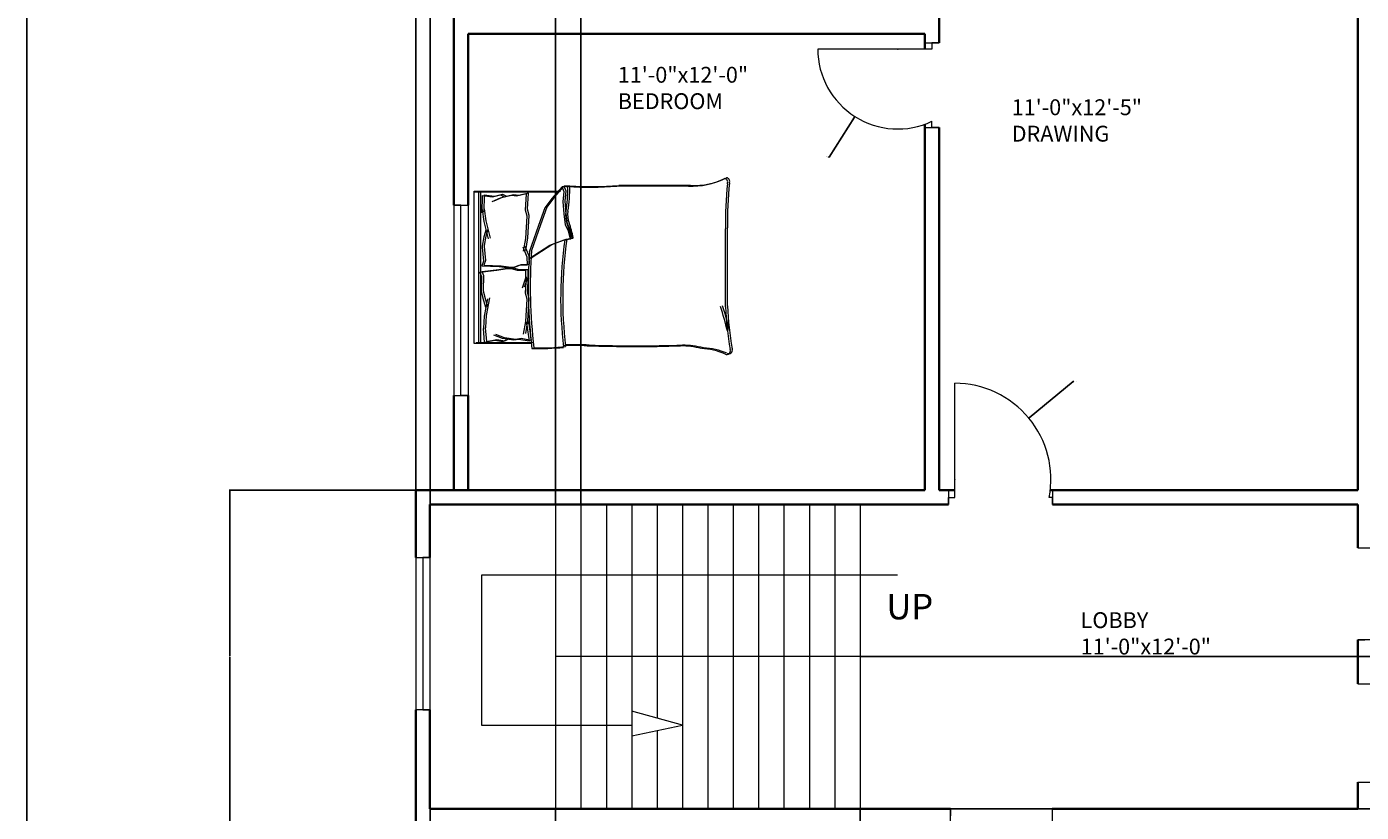
# Model space of a CAD drawing. Units: inches. Extents: x 2163 to 2982, y 1024 to 2288.
# Tile 9 of 22: x 2163 to 2583, y 1637 to 1885. Entities that reach past the tile are written whole.
import ezdxf

# ---------------------------------------------------------------- set-up
doc = ezdxf.new("R2010")
doc.units = ezdxf.units.IN
for name, color, linetype, lineweight in [('A-ANNO-DIMS', 2, 'Continuous', 18), ('A-ANNO-SYMB', 81, 'Continuous', 18), ('A-ANNO-TEXT', 7, 'Continuous', 18), ('A-ANNO-TTLB', 7, 'Continuous', 25), ('A-AREA-IDEN', 7, 'Continuous', 18), ('A-DOOR', 11, 'Continuous', 18), ('A-FLOR-STRS', 81, 'Continuous', 18), ('A-FURN', 8, 'Continuous', 13), ('A-GLAZ', 161, 'Continuous', 18), ('A-WALL', 7, 'Continuous', 35)]:
    doc.layers.add(name, color=color, linetype=linetype, lineweight=lineweight)
doc.styles.get("Standard").update_dxf_attribs({"font": 'arial.ttf'})
doc.dimstyles.get("Standard").update_dxf_attribs({"dimtxt": 0.18, "dimasz": 0.18, "dimexe": 0.18, "dimexo": 0.0625, "dimgap": 0.09, "dimtad": 0, "dimtih": 1, "dimtoh": 1, "dimdec": 4, "dimzin": 0, "dimdsep": 46, "dimtxsty": 'Standard', "dimcen": 0.09, "dimadec": 0, "dimazin": 0, "dimtfac": 1, "dimtdec": 4, "dimtofl": 0, "dimtmove": 0, "dimatfit": 3, "dimfxl": 1, "dimtolj": 1, "dimtzin": 0, "dimarcsym": 0})

# ---------------------------------------------------------------- blocks, each defined once
blk = doc.blocks.new('BED-DOUBLE')
for p, q in [((0, 51.49), (0.64, 51.49)), ((0, 3.47), (0, 51.49)), ((0, 51.27), (26.61, 51.27)), ((0, 51.27), (26.61, 51.27)), ((0.64, 51.49), (27.25, 51.49)), ((0.64, 51.49), (27.25, 51.49)), ((1.53, 3.48), (1.53, 51.27)), ((1.53, 3.47), (1.53, 51.27)), ((2.17, 3.7), (2.17, 51.49)), ((2.17, 3.7), (2.17, 51.49)), ((6.41, 49.96), (8.98, 50.56)), ((6.41, 49.96), (8.98, 50.56)), ((8.98, 50.56), (10.02, 50.04)), ((8.98, 50.56), (10.02, 50.04)), ((16.57, 50.7), (13.43, 49.92)), ((16.57, 50.7), (13.43, 49.92)), ((17.21, 50.93), (14.07, 50.15)), ((17.21, 50.93), (14.07, 50.15)), ((16.17, 45.57), (16.57, 50.7)), ((16.17, 45.57), (16.57, 50.7)), ((16.81, 45.79), (17.21, 50.93)), ((16.81, 45.79), (17.21, 50.93)), ((27.75, 52.87), (24.5, 49.16)), ((27.75, 52.87), (24.5, 49.16)), ((28.38, 53.1), (25.13, 49.39)), ((28.38, 53.1), (25.13, 49.39)), ((29.49, 52.95), (27.75, 52.87, 3.87)), ((29.49, 52.95), (27.75, 52.87, 3.87)), ((28.36, 51.33), (27.75, 52.87)), ((28.36, 51.33), (27.75, 52.87)), ((28.06, 48.23), (28.36, 51.33)), ((28.06, 48.23), (28.36, 51.33)), ((30.13, 53.18), (28.38, 53.1, 3.87)), ((29, 51.56), (28.38, 53.1)), ((30.13, 53.18), (28.38, 53.1, 3.87)), ((29, 51.56), (28.38, 53.1)), ((28.69, 48.46), (29, 51.56)), ((28.69, 48.46), (29, 51.56)), ((2.56, 50.11), (2.46, 44.71)), ((2.56, 50.11), (2.46, 44.71)), ((2.56, 50.11), (5.77, 49.73)), ((2.56, 50.11), (5.77, 49.73)), ((3.2, 50.34), (3.1, 44.94)), ((3.2, 50.34), (3.1, 44.94)), ((3.2, 50.34), (6.41, 49.96)), ((3.2, 50.34), (6.41, 49.96)), ((8.26, 49.31), (5.58, 48.13)), ((8.26, 49.31), (5.58, 48.13)), ((5.77, 49.73), (8.34, 50.33)), ((5.77, 49.73), (8.34, 50.33)), ((8.9, 49.54), (6.22, 48.36)), ((8.9, 49.54), (6.22, 48.36)), ((11.83, 50.11), (8.26, 49.31)), ((11.83, 50.11), (8.26, 49.31)), ((8.34, 50.33), (9.38, 49.81)), ((8.34, 50.33), (9.38, 49.81)), ((12.47, 50.34), (8.9, 49.54)), ((12.47, 50.34), (8.9, 49.54)), ((13.43, 49.92), (11.83, 50.11)), ((13.43, 49.92), (11.83, 50.11)), ((14.07, 50.15), (12.47, 50.34)), ((14.07, 50.15), (12.47, 50.34)), ((22.97, 46.45), (20.96, 40.87)), ((22.97, 46.45), (20.96, 40.87)), ((24.5, 49.16), (22.33, 46.22)), ((24.5, 49.16), (22.33, 46.22)), ((25.13, 49.39), (22.97, 46.45)), ((25.13, 49.39), (22.97, 46.45)), ((28.36, 44.36), (28.06, 48.23)), ((28.36, 44.36), (28.06, 48.23)), ((29, 44.59), (28.69, 48.46)), ((29, 44.59), (28.69, 48.46)), ((2.46, 44.71), (2.54, 45.71)), ((2.46, 44.71), (2.54, 45.71)), ((2.54, 45.71), (3.07, 41.91)), ((2.54, 45.71), (3.07, 41.91)), ((3.1, 44.94), (3.18, 45.94)), ((3.1, 44.94), (3.18, 45.94)), ((3.18, 45.94), (3.71, 42.14)), ((3.18, 45.94), (3.71, 42.14)), ((3.71, 42.14), (5.06, 36.72)), ((3.71, 42.14), (5.06, 36.72)), ((16.73, 43.61), (16.17, 45.57)), ((16.73, 43.61), (16.17, 45.57)), ((16.29, 36.6), (16.73, 43.61)), ((16.29, 36.6), (16.73, 43.61)), ((17.37, 43.83), (16.81, 45.79)), ((17.37, 43.83), (16.81, 45.79)), ((16.93, 36.82), (17.37, 43.83)), ((16.93, 36.82), (17.37, 43.83)), ((22.33, 46.22), (20.32, 40.64)), ((22.33, 46.22), (20.32, 40.64)), ((28.83, 40.95), (28.36, 44.36)), ((28.83, 40.95), (28.36, 44.36)), ((29.47, 41.18), (29, 44.59)), ((29.47, 41.18), (29, 44.59)), ((3.07, 41.91), (4.42, 36.49)), ((3.07, 41.91), (4.42, 36.49)), ((3.67, 39.2), (3.08, 37.14)), ((3.67, 39.2), (3.08, 37.13)), ((4.31, 39.43), (3.72, 37.36)), ((4.31, 39.43), (3.72, 37.36)), ((20.32, 40.64), (17.38, 32.31)), ((20.32, 40.64), (17.38, 32.31)), ((20.96, 40.87), (18.02, 32.53)), ((20.96, 40.87), (18.02, 32.53)), ((29.76, 38.94), (28.83, 40.95)), ((29.76, 38.94), (28.83, 40.95)), ((30.4, 39.17), (29.47, 41.18)), ((30.4, 39.17), (29.47, 41.18)), ((30.38, 36.46), (29.76, 38.94)), ((30.38, 36.46), (29.76, 38.94)), ((31.02, 36.69), (30.4, 39.17)), ((31.02, 36.69), (30.4, 39.17)), ((79.24, 15.06), (79.24, 39.68)), ((79.24, 15.06), (79.24, 39.68)), ((79.88, 15.29), (79.88, 39.91)), ((79.88, 15.29), (79.88, 39.91)), ((3.08, 37.14), (2.54, 34.2)), ((3.08, 37.13), (2.54, 34.2)), ((2.54, 34.2), (2.56, 33.88)), ((2.54, 34.2), (2.56, 33.88)), ((2.56, 33.88), (2.98, 29.46)), ((2.56, 33.88), (2.98, 29.46)), ((3.72, 37.36), (3.18, 34.43)), ((3.72, 37.36), (3.18, 34.43)), ((3.18, 34.43), (3.2, 34.11)), ((3.18, 34.43), (3.2, 34.11)), ((3.2, 34.11), (3.62, 29.68)), ((3.2, 34.11), (3.62, 29.68)), ((16.74, 30.75), (15.45, 33.82)), ((16.74, 30.75), (15.45, 33.82)), ((15.63, 32.56), (16.29, 36.6)), ((15.63, 32.56), (16.29, 36.6)), ((17.38, 30.98), (16.09, 34.05)), ((17.38, 30.98), (16.09, 34.05)), ((16.27, 32.79), (16.93, 36.82)), ((16.27, 32.79), (16.93, 36.82)), ((17.38, 30.26), (23.88, 34.45)), ((17.38, 30.26), (23.88, 34.45)), ((18.02, 30.49), (24.52, 34.68)), ((18.02, 30.49), (24.52, 34.68)), ((23.88, 34.45), (28.36, 36.15)), ((23.88, 34.45), (28.36, 36.15)), ((24.52, 34.68), (29, 36.38)), ((24.52, 34.68), (29, 36.38)), ((28.36, 36.15), (30.38, 36.46)), ((28.36, 36.15), (30.38, 36.46)), ((29, 36.38), (31.02, 36.69)), ((29, 36.38), (31.02, 36.69)), ((2.98, 29.46), (2.49, 27.98)), ((2.98, 29.46), (2.49, 27.98)), ((3.62, 29.68), (3.13, 28.21)), ((3.62, 29.68), (3.13, 28.2)), ((16.89, 28.3), (16.74, 30.75)), ((16.89, 28.3), (16.74, 30.75)), ((17.53, 28.53), (17.38, 30.98)), ((17.53, 28.53), (17.38, 30.98)), ((1.87, 25.98), (7.22, 26.56)), ((1.87, 25.98), (7.22, 26.56)), ((2.45, 24.54), (1.87, 25.98)), ((2.45, 24.54), (1.87, 25.98)), ((2.49, 27.98), (7.87, 27.73)), ((2.49, 27.98), (7.87, 27.73)), ((2.51, 26.21), (7.86, 26.79)), ((2.51, 26.21), (7.86, 26.79)), ((3.09, 24.77), (2.51, 26.21)), ((3.09, 24.77), (2.51, 26.21)), ((3.13, 28.21), (8.51, 27.96)), ((3.13, 28.2), (8.51, 27.96)), ((7.22, 26.56), (10.4, 27.14)), ((7.22, 26.56), (10.4, 27.14)), ((7.86, 26.79), (11.04, 27.37)), ((7.86, 26.79), (11.04, 27.37)), ((7.87, 27.73), (11.08, 27.35)), ((7.87, 27.73), (11.08, 27.35)), ((8.51, 27.96), (11.72, 27.58)), ((8.51, 27.96), (11.72, 27.58)), ((10.4, 27.14), (11.7, 27.14)), ((10.4, 27.14), (11.7, 27.14)), ((11.04, 27.37), (12.34, 27.37)), ((11.04, 27.37), (12.34, 27.37)), ((11.08, 27.35), (12.38, 27.44)), ((11.08, 27.35), (12.38, 27.44)), ((11.7, 27.14), (13.58, 26.56)), ((11.7, 27.14), (13.58, 26.56)), ((11.72, 27.58), (13.02, 27.66)), ((11.72, 27.58), (13.02, 27.66)), ((12.34, 27.37), (14.22, 26.79)), ((12.34, 27.37), (14.22, 26.79)), ((12.38, 27.44), (14.22, 28.13)), ((12.38, 27.44), (14.22, 28.13)), ((13.02, 27.66), (14.86, 28.36)), ((13.02, 27.66), (14.86, 28.36)), ((13.58, 26.56), (16.26, 26.56)), ((13.58, 26.56), (16.26, 26.56)), ((14.22, 28.13), (16.89, 28.3)), ((14.22, 28.13), (16.89, 28.3)), ((14.22, 26.79), (16.9, 26.79)), ((14.22, 26.79), (16.9, 26.79)), ((14.86, 28.36), (17.53, 28.53)), ((14.86, 28.36), (17.53, 28.53)), ((16.26, 26.56), (16.26, 24.1)), ((16.26, 26.56), (16.26, 24.1)), ((16.9, 26.79), (16.9, 24.33)), ((16.9, 26.79), (16.9, 24.33)), ((2.3, 20.09), (2.45, 24.54)), ((2.3, 20.09), (2.45, 24.54)), ((2.94, 20.32), (3.09, 24.77)), ((2.94, 20.32), (3.09, 24.77)), ((16.26, 24.1), (15.17, 20.96)), ((16.26, 24.1), (15.17, 20.96)), ((16.9, 24.33), (15.81, 21.19)), ((16.9, 24.33), (15.81, 21.19)), ((16.17, 19.38), (16.57, 24.52)), ((16.17, 19.38), (16.57, 24.52)), ((16.81, 19.61), (17.21, 24.74)), ((16.81, 19.61), (17.21, 24.74)), ((2.3, 19.77), (2.3, 20.09)), ((2.3, 19.77), (2.3, 20.09)), ((3.03, 16.88), (2.3, 19.77)), ((3.03, 16.88), (2.3, 19.77)), ((2.94, 20), (2.94, 20.32)), ((2.94, 20), (2.94, 20.32)), ((3.67, 17.11), (2.94, 20)), ((3.67, 17.11), (2.94, 20)), ((3.75, 14.85), (3.03, 16.88)), ((3.75, 14.85), (3.03, 16.88)), ((3.32, 12.11), (4.33, 17.6)), ((3.32, 12.11), (4.33, 17.6)), ((4.39, 15.08), (3.67, 17.11)), ((4.39, 15.08), (3.67, 17.11)), ((3.96, 12.34), (4.97, 17.83)), ((3.96, 12.34), (4.97, 17.83)), ((16.73, 17.42), (16.17, 19.38)), ((16.73, 17.42), (16.17, 19.38)), ((16.29, 10.41), (16.73, 17.42)), ((16.29, 10.41), (16.73, 17.42)), ((17.37, 17.65), (16.81, 19.61)), ((17.37, 17.65), (16.81, 19.61)), ((16.93, 10.64), (17.37, 17.65)), ((16.93, 10.64), (17.37, 17.65)), ((3.03, 8.28), (3.32, 12.11)), ((3.03, 8.28), (3.32, 12.11)), ((3.65, 8.41), (3.67, 8.51)), ((3.65, 8.41), (3.67, 8.51)), ((3.67, 8.51), (3.96, 12.34)), ((3.67, 8.51), (3.96, 12.34)), ((15.63, 6.38), (16.29, 10.41)), ((15.63, 6.38), (16.29, 10.41)), ((16.27, 6.61), (16.93, 10.64)), ((16.27, 6.61), (16.93, 10.64)), ((16.29, 10.41), (16.62, 9.28)), ((16.29, 10.41), (16.62, 9.28)), ((16.62, 9.28), (17.34, 4.18)), ((16.62, 9.28), (17.34, 4.18)), ((16.93, 10.64), (17.26, 9.51)), ((16.93, 10.64), (17.26, 9.51)), ((17.26, 9.51), (17.98, 4.41)), ((17.26, 9.51), (17.98, 4.41)), ((3.01, 8.18), (3.03, 8.28)), ((3.01, 8.18), (3.03, 8.28)), ((3.34, 3.9), (3.01, 8.18)), ((3.34, 3.9), (3.01, 8.18)), ((3.32, 3.89), (6.5, 4.47)), ((3.32, 3.89), (6.5, 4.47)), ((3.98, 4.13), (3.65, 8.41)), ((3.98, 4.13), (3.65, 8.41)), ((3.96, 4.12), (7.14, 4.7)), ((3.96, 4.12), (7.14, 4.7)), ((8.95, 5.05), (6.21, 6.06)), ((8.95, 5.05), (6.21, 6.06)), ((6.5, 4.47), (9.1, 4.04)), ((6.5, 4.47), (9.1, 4.04)), ((9.59, 5.28), (6.85, 6.29)), ((9.59, 5.28), (6.85, 6.29)), ((7.14, 4.7), (9.74, 4.27)), ((7.14, 4.7), (9.74, 4.27)), ((12.57, 4.47), (8.95, 5.05)), ((12.57, 4.47), (8.95, 5.05)), ((9.1, 4.04), (10.11, 4.62)), ((9.1, 4.04), (10.11, 4.62)), ((13.21, 4.7), (9.59, 5.28)), ((13.21, 4.7), (9.59, 5.28)), ((9.74, 4.27), (10.75, 4.85)), ((9.74, 4.27), (10.75, 4.85)), ((14.16, 4.76), (12.57, 4.47)), ((14.16, 4.76), (12.57, 4.47)), ((14.8, 4.99), (13.21, 4.7)), ((14.8, 4.99), (13.21, 4.7)), ((17.34, 4.18), (14.16, 4.76)), ((17.34, 4.18), (14.16, 4.76)), ((17.98, 4.41), (14.8, 4.99)), ((17.98, 4.41), (14.8, 4.99)), ((18.11, 3.48), (0, 3.48)), ((18.11, 3.47), (0, 3.47)), ((18.75, 3.7), (0.64, 3.7)), ((18.75, 3.7), (0.64, 3.7))]:
    blk.add_line(p, q)
for centre, radius, start, end in [((68.67, 76.16), 23.07, 267.4714, 296.4681), ((68.67, 76.16), 23.07, 267.4714, 296.4681), ((69.31, 76.39), 23.07, 267.4714, 296.4681), ((69.31, 76.39), 23.07, 267.4714, 296.4681), ((78.87, 54.41), 1.1, 332.6588, 86.02), ((78.87, 54.41), 1.1, 332.6588, 86.02), ((79.51, 54.64), 1.1, 332.6588, 86.02), ((79.51, 54.64), 1.1, 332.6588, 86.02), ((-6.66, 51.33), 36.18, 349.8763, 2.5657), ((-6.66, 51.33), 36.18, 349.8763, 2.5657), ((36.31, 182.27), 129.5, 266.9791, 273.8365), ((36.31, 182.27), 129.5, 266.9791, 273.8365), ((-6.02, 51.56), 36.18, 349.8763, 2.5657), ((-6.02, 51.56), 36.18, 349.8763, 2.5657), ((36.95, 182.49), 129.5, 266.9791, 273.8365), ((36.95, 182.49), 129.5, 266.9791, 273.8365), ((67.82, -4508.74), 4561.86, 90.00217, 90.28689), ((67.82, -4508.74), 4561.86, 90.00217, 90.28689), ((68.46, -4508.52), 4561.86, 90.00217, 90.28689), ((68.46, -4508.52), 4561.86, 90.00217, 90.28689), ((212.28, 41.15), 133.04, 174.4998, 180.6351), ((212.28, 41.15), 133.04, 174.4998, 180.6351), ((212.92, 41.38), 133.04, 174.4998, 180.6351), ((212.92, 41.38), 133.04, 174.4998, 180.6351), ((35.07, 43.74), 6.22, 168.6608, 203.7384), ((35.07, 43.74), 6.22, 168.6608, 203.7384), ((35.71, 43.97), 6.22, 168.6608, 203.7384), ((35.71, 43.97), 6.22, 168.6608, 203.7384), ((1.48, 31.15), 29.65, 10.6617, 19.8806), ((1.48, 31.15), 29.65, 10.6617, 19.8806), ((2.12, 31.38), 29.65, 10.6617, 19.8806), ((2.12, 31.38), 29.65, 10.6617, 19.8806), ((156.32, 17.76), 129.02, 171.7845, 186.9006), ((156.32, 17.76), 129.02, 171.7845, 186.9006), ((156.96, 17.98), 129.02, 171.7845, 186.9006), ((156.96, 17.98), 129.02, 171.7845, 186.9006), ((30.44, 36.64), 0.185, 250.2464, 1.1377), ((30.44, 36.64), 0.185, 250.2464, 1.1377), ((31.08, 36.86), 0.185, 250.2464, 1.1377), ((31.08, 36.86), 0.185, 250.2464, 1.1377), ((182.05, 21.36), 164.97, 176.0865, 186.7821), ((182.05, 21.36), 164.97, 176.0865, 186.7821), ((182.69, 21.59), 164.97, 176.0865, 186.7821), ((182.69, 21.59), 164.97, 176.0865, 186.7821), ((-23.71, -17.22), 106.46, 13.3832, 17.7053), ((-23.71, -17.22), 106.46, 13.3832, 17.7053), ((-23.07, -16.99), 106.46, 13.3832, 17.7053), ((-23.07, -16.99), 106.46, 13.3832, 17.7053), ((200.84, 21.43), 121.76, 182.9958, 189.4091), ((200.84, 21.43), 121.76, 182.9958, 189.4091), ((201.48, 21.66), 121.76, 182.9958, 189.4091), ((201.48, 21.65), 121.76, 182.9958, 189.4091), ((20.1, 85.16), 83.31, 268.7218, 275.604), ((20.1, 85.16), 83.31, 268.7218, 275.604), ((20.74, 85.39), 83.31, 268.7218, 275.604), ((20.74, 85.39), 83.31, 268.7218, 275.604), ((31.17, -167.31), 170.11, 88.4762, 91.0082), ((31.17, -167.31), 170.11, 88.4762, 91.0082), ((31.81, -167.08), 170.11, 88.4762, 91.0082), ((31.81, -167.08), 170.11, 88.4762, 91.0082), ((50.61, 484.82), 482.31, 268.2277, 271.7185), ((50.61, 484.82), 482.31, 268.2277, 271.7185), ((51.25, 485.05), 482.31, 268.2277, 271.7185), ((51.25, 485.05), 482.31, 268.2277, 271.7185), ((64.51, -26.9), 29.63, 76.0648, 88.9113), ((64.51, -26.9), 29.63, 76.0648, 88.9113), ((65.15, -26.67), 29.63, 76.0648, 88.9113), ((65.15, -26.67), 29.63, 76.0648, 88.9113), ((70.28, -21.66), 23.56, 67.9751, 86.652), ((70.28, -21.66), 23.56, 67.9751, 86.652), ((70.91, -21.43), 23.56, 67.9751, 86.652), ((70.91, -21.43), 23.56, 67.9751, 86.652), ((79.72, 1.09), 1.09, 236.1736, 23.4781), ((79.72, 1.09), 1.09, 236.1736, 23.4781), ((80.36, 1.32), 1.09, 236.1736, 23.4781), ((80.36, 1.32), 1.09, 236.1736, 23.4781)]:
    blk.add_arc(centre, radius, start, end)
blk = doc.blocks.new('WIN-60')
for p, q in [((2.25, 60), (0, 60)), ((0, 60), (4.5, 60)), ((0, 60), (0, 0)), ((2.25, 0), (2.25, 60)), ((4.5, 60), (4.5, 0)), ((0, 0), (4.5, 0)), ((4.5, 0), (2.25, 0))]:
    blk.add_line(p, q)
blk = doc.blocks.new('*D29')
at = {"layer": 'A-ANNO-DIMS', "color": 0, "lineweight": -2, "transparency": 16777216}
for p, q in [((2285.34, 1738.83), (2285.34, 2288.1)), ((2285.52, 2287.92), (2576.05, 2287.92)), ((2867.16, 2287.92), (2576.63, 2287.92)), ((2867.34, 2229.33), (2867.34, 2288.1))]:
    blk.add_line(p, q, dxfattribs=at)
at = {"layer": 'A-ANNO-DIMS', "color": 0, "transparency": 16777216}
for points in [[(2285.52, 2287.95), (2285.52, 2287.89), (2285.34, 2287.92)], [(2867.16, 2287.95), (2867.16, 2287.89), (2867.34, 2287.92)]]:
    blk.add_solid(points, dxfattribs=at)
at = {"layer": 'Defpoints', "color": 0, "transparency": 16777216}
for p in [(2867.34, 2287.92), (2867.34, 2229.27), (2285.34, 1738.77)]:
    blk.add_point(p, dxfattribs=at)
at = {"layer": 'A-ANNO-DIMS', "color": 0, "transparency": 16777216, "insert": (2576.34, 2287.92), "char_height": 0.18, "attachment_point": 5}
blk.add_mtext('\\A1;582', dxfattribs=at)
blk = doc.blocks.new('*D34')
at = {"layer": 'A-ANNO-DIMS', "color": 0, "lineweight": -2, "transparency": 16777216}
for p, q in [((2285.28, 1738.77), (2226.51, 1738.77)), ((2226.69, 1738.59), (2226.69, 1686.45)), ((2226.69, 1633.95), (2226.69, 1686.09)), ((2285.28, 1633.77), (2226.51, 1633.77))]:
    blk.add_line(p, q, dxfattribs=at)
at = {"layer": 'A-ANNO-DIMS', "color": 0, "transparency": 16777216}
for points in [[(2226.66, 1738.59), (2226.72, 1738.59), (2226.69, 1738.77)], [(2226.66, 1633.95), (2226.72, 1633.95), (2226.69, 1633.77)]]:
    blk.add_solid(points, dxfattribs=at)
at = {"layer": 'Defpoints', "color": 0, "transparency": 16777216}
for p in [(2226.69, 1738.77), (2285.34, 1738.77), (2285.34, 1633.77)]:
    blk.add_point(p, dxfattribs=at)
at = {"layer": 'A-ANNO-DIMS', "color": 0, "transparency": 16777216, "insert": (2226.69, 1686.27), "char_height": 0.18, "attachment_point": 5}
blk.add_mtext('\\A1;105', dxfattribs=at)
blk = doc.blocks.new('*D36')
at = {"layer": 'A-ANNO-DIMS', "color": 0, "lineweight": -2, "transparency": 16777216}
for p, q in [((2289.84, 1638.21), (2289.84, 1023.79)), ((2329.44, 1638.21), (2329.44, 1023.79)), ((2290.02, 1023.97), (2309.18, 1023.97)), ((2329.26, 1023.97), (2310.11, 1023.97))]:
    blk.add_line(p, q, dxfattribs=at)
at = {"layer": 'A-ANNO-DIMS', "color": 0, "transparency": 16777216}
for points in [[(2290.02, 1024), (2290.02, 1023.94), (2289.84, 1023.97)], [(2329.26, 1024), (2329.26, 1023.94), (2329.44, 1023.97)]]:
    blk.add_solid(points, dxfattribs=at)
at = {"layer": 'Defpoints', "color": 0, "transparency": 16777216}
for p in [(2289.84, 1638.27), (2329.44, 1638.27), (2329.44, 1023.97)]:
    blk.add_point(p, dxfattribs=at)
at = {"layer": 'A-ANNO-DIMS', "color": 0, "transparency": 16777216, "insert": (2309.64, 1023.97), "char_height": 0.18, "attachment_point": 5}
blk.add_mtext('\\A1;39.605', dxfattribs=at)
blk = doc.blocks.new('*D37')
at = {"layer": 'A-ANNO-DIMS', "color": 0, "lineweight": -2, "transparency": 16777216}
for p, q in [((2329.44, 1638.21), (2329.44, 1023.79)), ((2425.44, 1638.21), (2425.44, 1023.79)), ((2329.62, 1023.97), (2377.22, 1023.97)), ((2425.26, 1023.97), (2377.66, 1023.97))]:
    blk.add_line(p, q, dxfattribs=at)
at = {"layer": 'A-ANNO-DIMS', "color": 0, "transparency": 16777216}
for points in [[(2329.62, 1024), (2329.62, 1023.94), (2329.44, 1023.97)], [(2425.26, 1024), (2425.26, 1023.94), (2425.44, 1023.97)]]:
    blk.add_solid(points, dxfattribs=at)
at = {"layer": 'Defpoints', "color": 0, "transparency": 16777216}
for p in [(2329.44, 1638.27), (2425.44, 1638.27), (2425.44, 1023.97)]:
    blk.add_point(p, dxfattribs=at)
at = {"layer": 'A-ANNO-DIMS', "color": 0, "transparency": 16777216, "insert": (2377.44, 1023.97), "char_height": 0.18, "attachment_point": 5}
blk.add_mtext('\\A1;96', dxfattribs=at)
blk = doc.blocks.new('*D38')
at = {"layer": 'A-ANNO-DIMS', "color": 0, "lineweight": -2, "transparency": 16777216}
for p, q in [((2329.44, 1734.33), (2329.44, 2288.1)), ((2329.62, 2287.92), (2333.29, 2287.92)), ((2337.26, 2287.92), (2333.59, 2287.92)), ((2337.44, 1734.33), (2337.44, 2288.1))]:
    blk.add_line(p, q, dxfattribs=at)
at = {"layer": 'A-ANNO-DIMS', "color": 0, "transparency": 16777216}
for points in [[(2329.62, 2287.95), (2329.62, 2287.89), (2329.44, 2287.92)], [(2337.26, 2287.95), (2337.26, 2287.89), (2337.44, 2287.92)]]:
    blk.add_solid(points, dxfattribs=at)
at = {"layer": 'Defpoints', "color": 0, "transparency": 16777216}
for p in [(2337.44, 2287.92), (2329.44, 1734.27), (2337.44, 1734.27)]:
    blk.add_point(p, dxfattribs=at)
at = {"layer": 'A-ANNO-DIMS', "color": 0, "transparency": 16777216, "insert": (2333.44, 2287.92), "char_height": 0.18, "attachment_point": 5}
blk.add_mtext('\\A1;8', dxfattribs=at)
blk = doc.blocks.new('*D39')
at = {"layer": 'A-ANNO-DIMS', "color": 0, "lineweight": -2, "transparency": 16777216}
for p, q in [((2425.51, 1686.27), (2926.17, 1686.27)), ((2925.99, 1686.09), (2925.99, 1662.45)), ((2925.99, 1638.45), (2925.99, 1662.09)), ((2425.51, 1638.27), (2926.17, 1638.27))]:
    blk.add_line(p, q, dxfattribs=at)
at = {"layer": 'A-ANNO-DIMS', "color": 0, "transparency": 16777216}
for points in [[(2925.96, 1686.09), (2926.02, 1686.09), (2925.99, 1686.27)], [(2925.96, 1638.45), (2926.02, 1638.45), (2925.99, 1638.27)]]:
    blk.add_solid(points, dxfattribs=at)
at = {"layer": 'Defpoints', "color": 0, "transparency": 16777216}
for p in [(2425.44, 1686.27), (2925.99, 1686.27), (2425.44, 1638.27)]:
    blk.add_point(p, dxfattribs=at)
at = {"layer": 'A-ANNO-DIMS', "color": 0, "transparency": 16777216, "insert": (2925.99, 1662.27), "char_height": 0.18, "attachment_point": 5}
blk.add_mtext('\\A1;48', dxfattribs=at)
blk = doc.blocks.new('*D40')
at = {"layer": 'A-ANNO-DIMS', "color": 0, "lineweight": -2, "transparency": 16777216}
for p, q in [((2285.34, 1738.83), (2285.34, 2288.1)), ((2285.52, 2287.92), (2287.33, 2287.92)), ((2289.66, 2287.92), (2287.85, 2287.92)), ((2289.84, 1734.33), (2289.84, 2288.1))]:
    blk.add_line(p, q, dxfattribs=at)
at = {"layer": 'A-ANNO-DIMS', "color": 0, "transparency": 16777216}
for points in [[(2285.52, 2287.95), (2285.52, 2287.89), (2285.34, 2287.92)], [(2289.66, 2287.95), (2289.66, 2287.89), (2289.84, 2287.92)]]:
    blk.add_solid(points, dxfattribs=at)
at = {"layer": 'Defpoints', "color": 0, "transparency": 16777216}
for p in [(2289.84, 2287.92), (2285.34, 1738.77), (2289.84, 1734.27)]:
    blk.add_point(p, dxfattribs=at)
at = {"layer": 'A-ANNO-DIMS', "color": 0, "transparency": 16777216, "insert": (2287.59, 2287.92), "char_height": 0.18, "attachment_point": 5}
blk.add_mtext('\\A1;4.5', dxfattribs=at)
blk = doc.blocks.new('*D41')
at = {"layer": 'A-ANNO-DIMS', "color": 0, "lineweight": -2, "transparency": 16777216}
for p, q in [((2492.66, 1773.12), (2478.78, 1761.64)), ((2492.84, 1773.12), (2492.66, 1773.12)), ((2455.19, 1742.2), (2455.37, 1742.2)), ((2455.28, 1742.11), (2455.28, 1742.29))]:
    blk.add_line(p, q, dxfattribs=at)
at = {"layer": 'A-ANNO-DIMS', "color": 0, "transparency": 16777216}
blk.add_solid([(2478.76, 1761.66), (2478.8, 1761.62), (2478.64, 1761.53)], dxfattribs=at)
at = {"layer": 'Defpoints', "color": 0, "transparency": 16777216}
for p in [(2478.64, 1761.53), (2455.28, 1742.2)]:
    blk.add_point(p, dxfattribs=at)
at = {"layer": 'A-ANNO-DIMS', "color": 0, "transparency": 16777216, "insert": (2493.32, 1773.12), "char_height": 0.18, "attachment_point": 5}
blk.add_mtext('\\A1;R30.32', dxfattribs=at)
blk = doc.blocks.new('*D55')
at = {"layer": 'A-ANNO-DIMS', "color": 0, "lineweight": -2, "transparency": 16777216}
for p, q in [((2437.23, 1877.97), (2437.41, 1877.97)), ((2437.32, 1877.88), (2437.32, 1878.06)), ((2415.71, 1843.88), (2423.72, 1856.51)), ((2415.53, 1843.88), (2415.71, 1843.88))]:
    blk.add_line(p, q, dxfattribs=at)
at = {"layer": 'A-ANNO-DIMS', "color": 0, "transparency": 16777216}
blk.add_solid([(2423.69, 1856.53), (2423.74, 1856.49), (2423.81, 1856.66)], dxfattribs=at)
at = {"layer": 'Defpoints', "color": 0, "transparency": 16777216}
for p in [(2437.32, 1877.97), (2423.81, 1856.66)]:
    blk.add_point(p, dxfattribs=at)
at = {"layer": 'A-ANNO-DIMS', "color": 0, "transparency": 16777216, "insert": (2415.05, 1843.88), "char_height": 0.18, "attachment_point": 5}
blk.add_mtext('\\A1;R25.23', dxfattribs=at)

msp = doc.modelspace()

# ---------------------------------------------------------------- linework, layer by layer
at = {"layer": 'A-ANNO-SYMB'}
for p, q in [((2437.226, 1711.9357), (2306.0886, 1711.9357)), ((2306.0886, 1711.9357), (2306.0886, 1664.6807)), ((2369.4434, 1664.6807), (2353.4434, 1669.0665)), ((2353.4434, 1669.0665), (2353.4434, 1661.2519)), ((2306.0886, 1664.6807), (2353.4434, 1664.6807)), ((2353.4434, 1661.2519), (2369.4434, 1664.6807))]:
    msp.add_line(p, q, dxfattribs=at)
at = {"layer": 'A-ANNO-TTLB'}
msp.add_lwpolyline([(2162.6841, 2274.6054), (2982.469, 2274.6054), (2982.469, 1045.9691), (2162.6841, 1045.9691)], close=True, dxfattribs=at)
at = {"layer": 'A-DOOR'}
for p, q in [((2448.0889, 1877.973), (2412.0889, 1877.973)), ((2445.8389, 1879.973), (2450.3389, 1879.973)), ((2450.3389, 1879.973), (2448.0889, 1879.973)), ((2448.0889, 1879.973), (2448.0889, 1877.973)), ((2445.8389, 1853.158), (2450.3389, 1853.158)), ((2448.0889, 1853.158), (2448.0889, 1855.158)), ((2450.3389, 1853.158), (2448.0889, 1853.158)), ((2455.2792, 1736.5188), (2455.2792, 1772.5188)), ((2453.2792, 1738.7688), (2453.2792, 1734.2688)), ((2486.0647, 1738.7688), (2486.0647, 1734.2688)), ((2453.2792, 1734.2688), (2453.2792, 1736.5188)), ((2453.2792, 1736.5188), (2455.2792, 1736.5188)), ((2486.0647, 1736.5188), (2485.0647, 1736.5188)), ((2486.0647, 1734.2688), (2486.0647, 1736.5188)), ((2582.3389, 1720.5499), (2586.8389, 1720.5499)), ((2586.8389, 1691.5305), (2582.3389, 1691.5305)), ((2582.3389, 1691.5305), (2584.5889, 1691.5305)), ((2582.3389, 1677.6524), (2586.8389, 1677.6524)), ((2582.3389, 1646.614), (2586.8389, 1646.614)), ((2453.9219, 1633.7688), (2453.9219, 1638.2688)), ((2453.9219, 1638.2688), (2453.9219, 1636.0188)), ((2486.0038, 1638.2688), (2486.0038, 1633.7688))]:
    msp.add_line(p, q, dxfattribs=at)
for centre, radius, start, end in [((2437.3185, 1877.973), 25.2295, 180, 295.270891), ((2455.2792, 1742.1969), 30.3219, 349.207103, 90)]:
    msp.add_arc(centre, radius, start, end, dxfattribs=at)
at = {"layer": 'A-FLOR-STRS'}
for p, q in [((2329.4434, 1734.2688), (2329.4434, 1638.2688)), ((2337.4434, 1734.2688), (2337.4434, 1638.2688)), ((2345.4434, 1734.2688), (2345.4434, 1638.2688)), ((2353.4434, 1734.2688), (2353.4434, 1638.2688)), ((2361.4434, 1734.2688), (2361.4434, 1666.8736)), ((2369.4434, 1734.2688), (2369.4434, 1638.2688)), ((2377.4434, 1734.2688), (2377.4434, 1638.2688)), ((2385.4434, 1734.2688), (2385.4434, 1638.2688)), ((2393.4434, 1734.2688), (2393.4434, 1638.2688)), ((2401.4434, 1734.2688), (2401.4434, 1638.2688)), ((2409.4434, 1734.2688), (2409.4434, 1638.2688)), ((2417.4434, 1734.2688), (2417.4434, 1638.2688)), ((2425.4434, 1734.2688), (2425.4434, 1638.2688)), ((2425.4434, 1686.2688), (2329.4434, 1686.2688)), ((2361.4434, 1662.9663), (2361.4434, 1638.2688))]:
    msp.add_line(p, q, dxfattribs=at)
at = {"layer": 'A-GLAZ'}
for p, q in [((2285.3389, 1717.5085), (2289.8389, 1717.5085)), ((2285.3389, 1717.5085), (2285.3389, 1669.5085)), ((2289.8389, 1717.5085), (2287.5889, 1717.5085)), ((2287.5889, 1717.5085), (2287.5889, 1669.5085)), ((2289.8389, 1717.5085), (2289.8389, 1669.5085)), ((2289.8389, 1669.5085), (2285.3389, 1669.5085)), ((2287.5889, 1669.5085), (2289.8389, 1669.5085))]:
    msp.add_line(p, q, dxfattribs=at)
at = {"layer": 'A-WALL'}
for p, q in [((2582.3389, 2011.7688), (2582.3389, 1738.7688)), ((2450.3389, 1963.7688), (2450.3389, 1879.973)), ((2297.3389, 1911.3655), (2297.3389, 1828.6523)), ((2301.8389, 1882.7688), (2445.8389, 1882.7688)), ((2301.8389, 1882.7688), (2301.8389, 1828.6523)), ((2445.8389, 1882.7688), (2445.8389, 1877.973)), ((2445.8389, 1854.2258), (2445.8389, 1738.7688)), ((2450.3389, 1853.158), (2450.3389, 1738.7688)), ((2297.3389, 1768.6523), (2297.3389, 1738.7688)), ((2301.8389, 1768.6523), (2301.8389, 1738.7688)), ((2297.3389, 1738.7688), (2285.3389, 1738.7688)), ((2285.3389, 1738.7688), (2285.3389, 1717.5085)), ((2301.8389, 1738.7688), (2297.3389, 1738.7688)), ((2301.8389, 1738.7688), (2445.8389, 1738.7688)), ((2450.3389, 1738.7688), (2455.2792, 1738.7688)), ((2485.4067, 1738.7688), (2582.3389, 1738.7688)), ((2289.8389, 1734.2688), (2301.8389, 1734.2688)), ((2289.8389, 1717.5085), (2289.8389, 1734.2688)), ((2301.8389, 1734.2688), (2453.2792, 1734.2688)), ((2486.0647, 1734.2688), (2582.3389, 1734.2688)), ((2582.3389, 1734.2688), (2582.3389, 1720.5499)), ((2582.3389, 1691.5305), (2582.3389, 1677.6524)), ((2285.3389, 1669.5085), (2285.3389, 1633.7688)), ((2289.8389, 1638.2688), (2289.8389, 1669.5085)), ((2582.3389, 1646.614), (2582.3389, 1638.2688)), ((2301.8389, 1638.2688), (2289.8389, 1638.2688)), ((2301.8389, 1638.2688), (2453.9219, 1638.2688)), ((2486.0038, 1638.2688), (2582.3389, 1638.2688))]:
    msp.add_line(p, q, dxfattribs=at)

# ---------------------------------------------------------------- block references
at = {"layer": 'A-FURN'}
msp.add_blockref('BED-DOUBLE', (2303.7323, 1781.5998), dxfattribs=at)
at = {"layer": 'A-GLAZ'}
msp.add_blockref('WIN-60', (2297.339, 1768.6523), dxfattribs=at)

# ---------------------------------------------------------------- texts
at = {"layer": 'A-ANNO-TEXT', "insert": (2433.7071, 1706.0278), "char_height": 8, "attachment_point": 1, "line_spacing_factor": 2.16}
msp.add_mtext_dynamic_manual_height_columns('UP', width=38.702945, gutter_width=12.5, heights=[0], dxfattribs=at)
at = {"layer": 'A-AREA-IDEN', "char_height": 5, "attachment_point": 1}
for s, width, insert in [('11\'-0"x12\'-0"\\PBEDROOM', 85.185595, (2349.0372, 1872.3442)), ('11\'-0"x12\'-5"\\PDRAWING', 87.474442, (2473.2272, 1862.0982)), ('LOBBY\\P11\'-0"x12\'-0"', 52.795421, (2494.9638, 1700.2763))]:
    msp.add_mtext_dynamic_manual_height_columns(s, width=width, gutter_width=12.5, heights=[0], dxfattribs=dict(at, insert=insert))

# ---------------------------------------------------------------- dimensions: what is measured, and where the dimension line sits
at = {"layer": 'A-ANNO-DIMS'}
for base, p1, p2, override, picture, middle in [((2867.3389, 2287.9188), (2285.3389, 1738.7688), (2867.3389, 2229.2688), {"dimdec": 0, "dimlfac": 1, "dimrnd": 0, "dimzin": 0, "dimdsep": 46, "dimlunit": 2}, '*D29', (2576.3389, 2287.9188)), ((2289.8389, 2287.9188), (2285.3389, 1738.7688), (2289.8389, 1734.2688), {"dimdec": 1, "dimlfac": 1, "dimrnd": 0, "dimzin": 0, "dimdsep": 46, "dimlunit": 2}, '*D40', (2287.5889, 2287.9188)), ((2337.4434, 2287.9188), (2329.4434, 1734.2688), (2337.4434, 1734.2688), {"dimdec": 0, "dimlfac": 1, "dimrnd": 0, "dimzin": 0, "dimdsep": 46, "dimlunit": 2}, '*D38', (2333.4434, 2287.9188)), ((2329.44344, 1023.97342), (2289.83891, 1638.26884), (2329.44344, 1638.26884), {"dimdec": 3, "dimlfac": 1, "dimrnd": 0, "dimzin": 0, "dimdsep": 46, "dimlunit": 2}, '*D36', (2309.64118, 1023.97342)), ((2425.4434, 1023.9734), (2329.4434, 1638.2688), (2425.4434, 1638.2688), {"dimdec": 0, "dimlfac": 1, "dimrnd": 0, "dimzin": 0, "dimdsep": 46, "dimlunit": 2}, '*D37', (2377.4434, 1023.9734))]:
    dim = msp.add_linear_dim(base=base, p1=p1, p2=p2, dimstyle='Standard', override=override, dxfattribs=at)
    dim.commit()
    dim.dimension.update_dxf_attribs({"geometry": picture, "text_midpoint": middle})
for center, mpoint, picture, middle in [((2437.3185, 1877.973), (2423.8128, 1856.6627), '*D55', (2415.0496, 1843.8766)), ((2455.2792, 1742.1969), (2478.6414, 1761.5263), '*D41', (2493.3176, 1773.124))]:
    dim = msp.add_radius_dim(center=center, mpoint=mpoint, dimstyle='Standard', override={"dimdec": 2, "dimlfac": 1, "dimrnd": 0, "dimzin": 0, "dimdsep": 46, "dimlunit": 2}, dxfattribs=at)
    dim.commit()
    dim.dimension.update_dxf_attribs({"geometry": picture, "text_midpoint": middle, "dimtype": 164})
for base, p1, p2, picture, middle in [((2226.6889, 1738.7688), (2285.3389, 1633.7688), (2285.3389, 1738.7688), '*D34', (2226.6889, 1686.2688)), ((2925.9889, 1686.2688), (2425.4434, 1638.2688), (2425.4434, 1686.2688), '*D39', (2925.9889, 1662.2688))]:
    dim = msp.add_linear_dim(base=base, p1=p1, p2=p2, angle=90, dimstyle='Standard', override={"dimdec": 0, "dimlfac": 1, "dimrnd": 0, "dimzin": 0, "dimdsep": 46, "dimlunit": 2}, dxfattribs=at)
    dim.commit()
    dim.dimension.update_dxf_attribs({"geometry": picture, "text_midpoint": middle})

doc.saveas('drawing.dxf')
